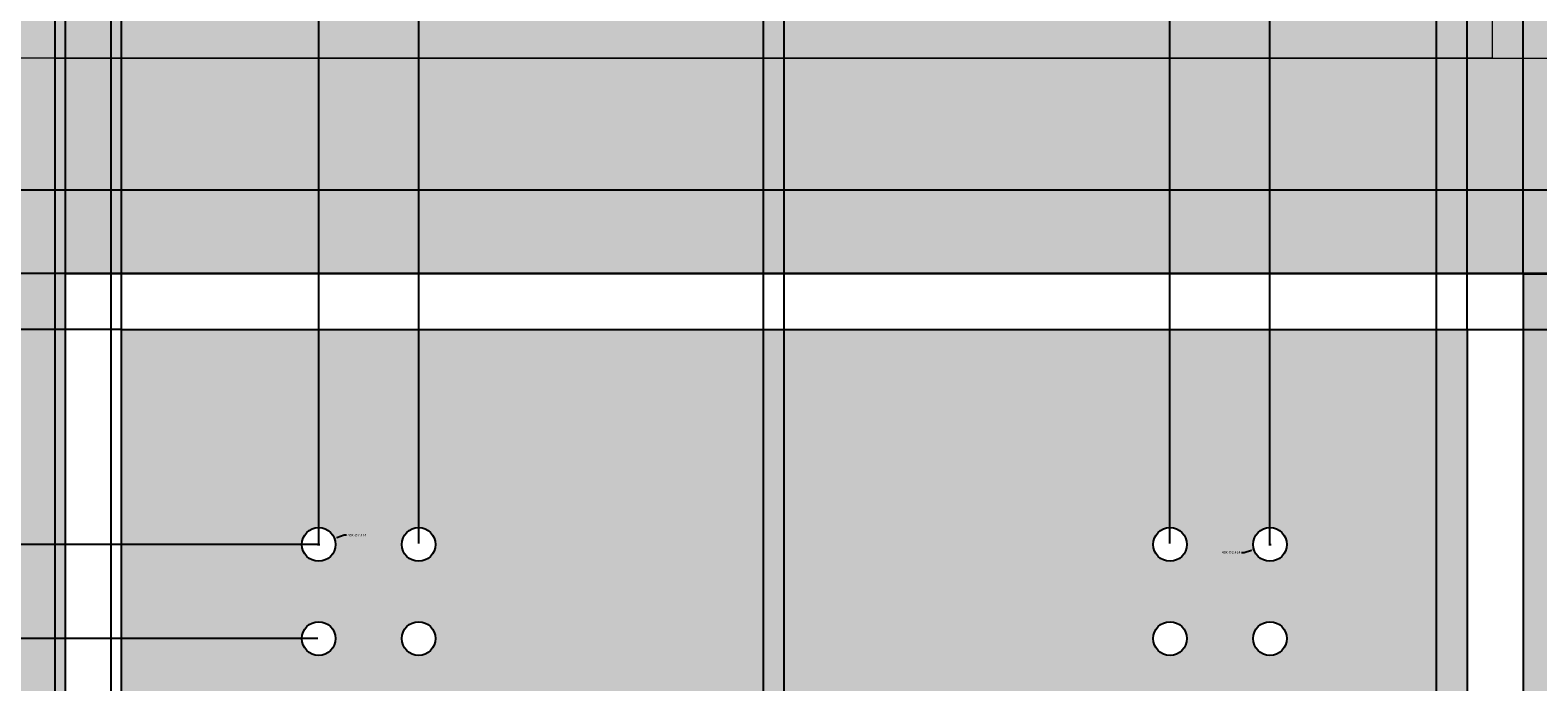
# Model space of a CAD drawing. Units: inches. Extents: x 3024 to 4744, y 1110 to 2100.
# Tile 6 of 29: x 3168 to 3275, y 1246 to 1293. Entities that reach past the tile are written whole.
import ezdxf

# ---------------------------------------------------------------- set-up
doc = ezdxf.new("R2010")
doc.units = ezdxf.units.IN
for name, color, linetype, lineweight in [('A-ANNO-DIMS', 2, 'Continuous', 18), ('A-ELEV', 7, 'Continuous', 25), ('A-ELEV-PATT', 252, 'Continuous', 13), ('A-GLAZ', 4, 'Continuous', 18)]:
    doc.layers.add(name, color=color, linetype=linetype, lineweight=lineweight)
doc.styles.get("Standard").update_dxf_attribs({"font": 'arial.ttf'})
doc.dimstyles.get("Standard").update_dxf_attribs({"dimtxt": 0.18, "dimasz": 0.18, "dimexe": 0.18, "dimexo": 0.0625, "dimgap": 0.09, "dimtad": 0, "dimtih": 1, "dimtoh": 1, "dimdec": 1, "dimzin": 0, "dimdsep": 46, "dimlunit": 3, "dimtxsty": 'Standard', "dimcen": 0.09, "dimadec": 0, "dimazin": 0, "dimtfac": 1, "dimtdec": 1, "dimtofl": 0, "dimtmove": 0, "dimatfit": 3, "dimfxl": 1, "dimtolj": 1, "dimtzin": 0, "dimarcsym": 0})

# ---------------------------------------------------------------- blocks, each defined once
blk = doc.blocks.new('WIN-BALCONY-A')
for q in [(3148.97, 1795.04), (3148.97, 1795.04), (3292.61, 1795.04), (3292.61, 1795.04)]:
    blk.add_line((3169.4, 1795.04), q)
blk.add_lwpolyline([(3272.18, 1795.04), (3169.4, 1795.04), (3169.4, 1897.49), (3272.18, 1897.49)], close=True)
blk.add_lwpolyline([(3272.18, 1795.04), (3169.4, 1795.04), (3169.4, 1897.49), (3272.18, 1897.49)], close=True)
blk.add_lwpolyline([(3292.61, 1795.04), (3292.61, 1785.61), (3148.97, 1785.61), (3148.97, 1795.04)])
blk.add_lwpolyline([(3292.61, 1795.04), (3292.61, 1785.61), (3148.97, 1785.61), (3148.97, 1795.04)])
blk = doc.blocks.new('*D52')
at = {"layer": 'A-ANNO-DIMS', "color": 0, "lineweight": -2, "transparency": 16777216}
for p, q in [((3148.97, 1290.98), (3148.97, 1109.93)), ((3170.16, 1170.96), (3170.16, 1109.93)), ((3149.15, 1110.11), (3159.17, 1110.11)), ((3169.98, 1110.11), (3159.96, 1110.11))]:
    blk.add_line(p, q, dxfattribs=at)
at = {"layer": 'A-ANNO-DIMS', "color": 0, "transparency": 16777216}
for points in [[(3149.15, 1110.14), (3149.15, 1110.08), (3148.97, 1110.11)], [(3169.98, 1110.14), (3169.98, 1110.08), (3170.16, 1110.11)]]:
    blk.add_solid(points, dxfattribs=at)
at = {"layer": 'Defpoints', "color": 0, "transparency": 16777216}
for p in [(3148.97, 1291.04), (3170.16, 1171.02), (3170.16, 1110.11)]:
    blk.add_point(p, dxfattribs=at)
at = {"layer": 'A-ANNO-DIMS', "color": 0, "transparency": 16777216, "insert": (3159.57, 1110.11), "char_height": 0.18, "attachment_point": 5}
blk.add_mtext('\\A1;21.19', dxfattribs=at)
blk = doc.blocks.new('*D54')
at = {"layer": 'A-ANNO-DIMS', "color": 0, "lineweight": -2, "transparency": 16777216}
for p, q in [((3292.61, 1290.98), (3292.61, 1109.93)), ((3274.39, 1170.96), (3274.39, 1109.93)), ((3274.57, 1110.11), (3283.04, 1110.11)), ((3292.43, 1110.11), (3283.95, 1110.11))]:
    blk.add_line(p, q, dxfattribs=at)
at = {"layer": 'A-ANNO-DIMS', "color": 0, "transparency": 16777216}
for points in [[(3274.57, 1110.14), (3274.57, 1110.08), (3274.39, 1110.11)], [(3292.43, 1110.14), (3292.43, 1110.08), (3292.61, 1110.11)]]:
    blk.add_solid(points, dxfattribs=at)
at = {"layer": 'Defpoints', "color": 0, "transparency": 16777216}
for p in [(3292.61, 1291.04), (3274.39, 1171.02), (3292.61, 1110.11)]:
    blk.add_point(p, dxfattribs=at)
at = {"layer": 'A-ANNO-DIMS', "color": 0, "transparency": 16777216, "insert": (3283.5, 1110.11), "char_height": 0.18, "attachment_point": 5}
blk.add_mtext('\\A1;18.217', dxfattribs=at)
blk = doc.blocks.new('*D64')
at = {"layer": 'A-ANNO-DIMS', "color": 0, "lineweight": -2, "transparency": 16777216}
for p, q in [((3069.79, 1241.5), (3069.79, 2100.44)), ((3741.15, 1241.5), (3741.15, 2100.44)), ((3069.97, 2100.26), (3405.08, 2100.26)), ((3740.97, 2100.26), (3405.87, 2100.26))]:
    blk.add_line(p, q, dxfattribs=at)
at = {"layer": 'A-ANNO-DIMS', "color": 0, "transparency": 16777216}
for points in [[(3069.97, 2100.29), (3069.97, 2100.23), (3069.79, 2100.26)], [(3740.97, 2100.29), (3740.97, 2100.23), (3741.15, 2100.26)]]:
    blk.add_solid(points, dxfattribs=at)
at = {"layer": 'Defpoints', "color": 0, "transparency": 16777216}
for p in [(3741.15, 2100.26), (3069.79, 1241.43), (3741.15, 1241.43)]:
    blk.add_point(p, dxfattribs=at)
at = {"layer": 'A-ANNO-DIMS', "color": 0, "transparency": 16777216, "insert": (3405.47, 2100.26), "char_height": 0.18, "attachment_point": 5}
blk.add_mtext('\\A1;671.4', dxfattribs=at)
blk = doc.blocks.new('*D77')
at = {"layer": 'A-ANNO-DIMS', "color": 0, "lineweight": -2, "transparency": 16777216}
for p, q in [((3188.17, 1256.23), (3188.35, 1256.23)), ((3188.26, 1256.14), (3188.26, 1256.32)), ((3190.07, 1256.89), (3189.56, 1256.71)), ((3190.25, 1256.89), (3190.07, 1256.89))]:
    blk.add_line(p, q, dxfattribs=at)
at = {"layer": 'A-ANNO-DIMS', "color": 0, "transparency": 16777216}
blk.add_solid([(3189.55, 1256.73), (3189.57, 1256.68), (3189.39, 1256.64)], dxfattribs=at)
at = {"layer": 'Defpoints', "color": 0, "transparency": 16777216}
for p in [(3189.39, 1256.64), (3187.13, 1255.81)]:
    blk.add_point(p, dxfattribs=at)
at = {"layer": 'A-ANNO-DIMS', "color": 0, "transparency": 16777216, "insert": (3191, 1256.89), "char_height": 0.18, "attachment_point": 5}
blk.add_mtext('\\A1;40X ∅2.414', dxfattribs=at)
blk = doc.blocks.new('*D90')
at = {"layer": 'A-ANNO-DIMS', "color": 0, "lineweight": -2, "transparency": 16777216}
for p, q in [((3173.4, 1798.98), (3173.4, 1109.93)), ((3169.4, 1794.98), (3169.4, 1109.93)), ((3169.58, 1110.11), (3171.07, 1110.11)), ((3173.22, 1110.11), (3171.72, 1110.11))]:
    blk.add_line(p, q, dxfattribs=at)
at = {"layer": 'A-ANNO-DIMS', "color": 0, "transparency": 16777216}
for points in [[(3169.58, 1110.14), (3169.58, 1110.08), (3169.4, 1110.11)], [(3173.22, 1110.14), (3173.22, 1110.08), (3173.4, 1110.11)]]:
    blk.add_solid(points, dxfattribs=at)
at = {"layer": 'Defpoints', "color": 0, "transparency": 16777216}
for p in [(3173.4, 1799.04), (3169.4, 1795.04), (3173.4, 1110.11)]:
    blk.add_point(p, dxfattribs=at)
at = {"layer": 'A-ANNO-DIMS', "color": 0, "transparency": 16777216, "insert": (3171.4, 1110.11), "char_height": 0.18, "attachment_point": 5}
blk.add_mtext('\\A1;4.00', dxfattribs=at)
blk = doc.blocks.new('*D91')
at = {"layer": 'A-ANNO-DIMS', "color": 0, "lineweight": -2, "transparency": 16777216}
for p, q in [((3173.4, 1798.98), (3173.4, 1109.93)), ((3220.05, 1798.98), (3220.05, 1109.93)), ((3173.58, 1110.11), (3196.33, 1110.11)), ((3219.87, 1110.11), (3197.12, 1110.11))]:
    blk.add_line(p, q, dxfattribs=at)
at = {"layer": 'A-ANNO-DIMS', "color": 0, "transparency": 16777216}
for points in [[(3173.58, 1110.14), (3173.58, 1110.08), (3173.4, 1110.11)], [(3219.87, 1110.14), (3219.87, 1110.08), (3220.05, 1110.11)]]:
    blk.add_solid(points, dxfattribs=at)
at = {"layer": 'Defpoints', "color": 0, "transparency": 16777216}
for p in [(3173.4, 1799.04), (3220.05, 1799.04), (3220.05, 1110.11)]:
    blk.add_point(p, dxfattribs=at)
at = {"layer": 'A-ANNO-DIMS', "color": 0, "transparency": 16777216, "insert": (3196.72, 1110.11), "char_height": 0.18, "attachment_point": 5}
blk.add_mtext('\\A1;46.65', dxfattribs=at)
blk = doc.blocks.new('*D92')
at = {"layer": 'A-ANNO-DIMS', "color": 0, "lineweight": -2, "transparency": 16777216}
for p, q in [((3220.05, 1798.98), (3220.05, 1109.93)), ((3221.52, 1798.98), (3221.52, 1109.93)), ((3220.23, 1110.11), (3220.47, 1110.11)), ((3221.34, 1110.11), (3221.1, 1110.11))]:
    blk.add_line(p, q, dxfattribs=at)
at = {"layer": 'A-ANNO-DIMS', "color": 0, "transparency": 16777216}
for points in [[(3220.23, 1110.14), (3220.23, 1110.08), (3220.05, 1110.11)], [(3221.34, 1110.14), (3221.34, 1110.08), (3221.52, 1110.11)]]:
    blk.add_solid(points, dxfattribs=at)
at = {"layer": 'Defpoints', "color": 0, "transparency": 16777216}
for p in [(3220.05, 1799.04), (3221.52, 1799.04), (3221.52, 1110.11)]:
    blk.add_point(p, dxfattribs=at)
at = {"layer": 'A-ANNO-DIMS', "color": 0, "transparency": 16777216, "insert": (3220.79, 1110.11), "char_height": 0.18, "attachment_point": 5}
blk.add_mtext('\\A1;1.47', dxfattribs=at)
blk = doc.blocks.new('*D93')
at = {"layer": 'A-ANNO-DIMS', "color": 0, "lineweight": -2, "transparency": 16777216}
for p, q in [((3221.52, 1798.98), (3221.52, 1109.93)), ((3268.18, 1798.98), (3268.18, 1109.93)), ((3221.7, 1110.11), (3244.45, 1110.11)), ((3268, 1110.11), (3245.25, 1110.11))]:
    blk.add_line(p, q, dxfattribs=at)
at = {"layer": 'A-ANNO-DIMS', "color": 0, "transparency": 16777216}
for points in [[(3221.7, 1110.14), (3221.7, 1110.08), (3221.52, 1110.11)], [(3268, 1110.14), (3268, 1110.08), (3268.18, 1110.11)]]:
    blk.add_solid(points, dxfattribs=at)
at = {"layer": 'Defpoints', "color": 0, "transparency": 16777216}
for p in [(3221.52, 1799.04), (3268.18, 1799.04), (3268.18, 1110.11)]:
    blk.add_point(p, dxfattribs=at)
at = {"layer": 'A-ANNO-DIMS', "color": 0, "transparency": 16777216, "insert": (3244.85, 1110.11), "char_height": 0.18, "attachment_point": 5}
blk.add_mtext('\\A1;46.65', dxfattribs=at)
blk = doc.blocks.new('*D106')
at = {"layer": 'A-ANNO-DIMS', "color": 0, "lineweight": -2, "transparency": 16777216}
for p, q in [((3170.16, 1275.67), (3170.16, 2100.44)), ((3174.16, 1271.67), (3174.16, 2100.44)), ((3170.34, 2100.26), (3171.83, 2100.26)), ((3173.98, 2100.26), (3172.49, 2100.26))]:
    blk.add_line(p, q, dxfattribs=at)
at = {"layer": 'A-ANNO-DIMS', "color": 0, "transparency": 16777216}
for points in [[(3170.34, 2100.29), (3170.34, 2100.23), (3170.16, 2100.26)], [(3173.98, 2100.29), (3173.98, 2100.23), (3174.16, 2100.26)]]:
    blk.add_solid(points, dxfattribs=at)
at = {"layer": 'Defpoints', "color": 0, "transparency": 16777216}
for p in [(3174.16, 2100.26), (3170.16, 1275.61), (3174.16, 1271.61)]:
    blk.add_point(p, dxfattribs=at)
at = {"layer": 'A-ANNO-DIMS', "color": 0, "transparency": 16777216, "insert": (3172.16, 2100.26), "char_height": 0.18, "attachment_point": 5}
blk.add_mtext('\\A1;4.00', dxfattribs=at)
blk = doc.blocks.new('*D107')
at = {"layer": 'A-ANNO-DIMS', "color": 0, "lineweight": -2, "transparency": 16777216}
for p, q in [((3174.16, 1271.67), (3174.16, 2100.44)), ((3270.39, 1271.67), (3270.39, 2100.44)), ((3174.34, 2100.26), (3221.88, 2100.26)), ((3270.21, 2100.26), (3222.67, 2100.26))]:
    blk.add_line(p, q, dxfattribs=at)
at = {"layer": 'A-ANNO-DIMS', "color": 0, "transparency": 16777216}
for points in [[(3174.34, 2100.29), (3174.34, 2100.23), (3174.16, 2100.26)], [(3270.21, 2100.29), (3270.21, 2100.23), (3270.39, 2100.26)]]:
    blk.add_solid(points, dxfattribs=at)
at = {"layer": 'Defpoints', "color": 0, "transparency": 16777216}
for p in [(3270.39, 2100.26), (3174.16, 1271.61), (3270.39, 1271.61)]:
    blk.add_point(p, dxfattribs=at)
at = {"layer": 'A-ANNO-DIMS', "color": 0, "transparency": 16777216, "insert": (3222.27, 2100.26), "char_height": 0.18, "attachment_point": 5}
blk.add_mtext('\\A1;96.23', dxfattribs=at)
blk = doc.blocks.new('*D108')
at = {"layer": 'A-ANNO-DIMS', "color": 0, "lineweight": -2, "transparency": 16777216}
for p, q in [((3270.39, 1271.67), (3270.39, 2100.44)), ((3274.39, 1275.67), (3274.39, 2100.44)), ((3270.57, 2100.26), (3272.06, 2100.26)), ((3274.21, 2100.26), (3272.71, 2100.26))]:
    blk.add_line(p, q, dxfattribs=at)
at = {"layer": 'A-ANNO-DIMS', "color": 0, "transparency": 16777216}
for points in [[(3270.57, 2100.29), (3270.57, 2100.23), (3270.39, 2100.26)], [(3274.21, 2100.29), (3274.21, 2100.23), (3274.39, 2100.26)]]:
    blk.add_solid(points, dxfattribs=at)
at = {"layer": 'Defpoints', "color": 0, "transparency": 16777216}
for p in [(3274.39, 2100.26), (3274.39, 1275.61), (3270.39, 1271.61)]:
    blk.add_point(p, dxfattribs=at)
at = {"layer": 'A-ANNO-DIMS', "color": 0, "transparency": 16777216, "insert": (3272.39, 2100.26), "char_height": 0.18, "attachment_point": 5}
blk.add_mtext('\\A1;4.00', dxfattribs=at)
blk = doc.blocks.new('*D120')
at = {"layer": 'A-ANNO-DIMS', "color": 0, "lineweight": -2, "transparency": 16777216}
for p, q in [((3270.45, 1271.61), (3786.83, 1271.61)), ((3786.65, 1271.43), (3786.65, 1221.5)), ((3786.65, 1171.2), (3786.65, 1221.14)), ((3274.45, 1171.02), (3786.83, 1171.02))]:
    blk.add_line(p, q, dxfattribs=at)
at = {"layer": 'A-ANNO-DIMS', "color": 0, "transparency": 16777216}
for points in [[(3786.62, 1271.43), (3786.68, 1271.43), (3786.65, 1271.61)], [(3786.62, 1171.2), (3786.68, 1171.2), (3786.65, 1171.02)]]:
    blk.add_solid(points, dxfattribs=at)
at = {"layer": 'Defpoints', "color": 0, "transparency": 16777216}
for p in [(3270.39, 1271.61), (3786.65, 1271.61), (3274.39, 1171.02)]:
    blk.add_point(p, dxfattribs=at)
at = {"layer": 'A-ANNO-DIMS', "color": 0, "transparency": 16777216, "insert": (3786.65, 1221.32), "char_height": 0.18, "attachment_point": 5}
blk.add_mtext('\\A1;100.59', dxfattribs=at)
blk = doc.blocks.new('*D121')
at = {"layer": 'A-ANNO-DIMS', "color": 0, "lineweight": -2, "transparency": 16777216}
for p, q in [((3274.45, 1275.61), (3786.83, 1275.61)), ((3786.65, 1275.43), (3786.65, 1273.79)), ((3786.65, 1271.79), (3786.65, 1273.43)), ((3270.45, 1271.61), (3786.83, 1271.61))]:
    blk.add_line(p, q, dxfattribs=at)
at = {"layer": 'A-ANNO-DIMS', "color": 0, "transparency": 16777216}
for points in [[(3786.62, 1275.43), (3786.68, 1275.43), (3786.65, 1275.61)], [(3786.62, 1271.79), (3786.68, 1271.79), (3786.65, 1271.61)]]:
    blk.add_solid(points, dxfattribs=at)
at = {"layer": 'Defpoints', "color": 0, "transparency": 16777216}
for p in [(3274.39, 1275.61), (3786.65, 1275.61), (3270.39, 1271.61)]:
    blk.add_point(p, dxfattribs=at)
at = {"layer": 'A-ANNO-DIMS', "color": 0, "transparency": 16777216, "insert": (3786.65, 1273.61), "char_height": 0.18, "attachment_point": 5}
blk.add_mtext('\\A1;4.00', dxfattribs=at)
blk = doc.blocks.new('*D124')
at = {"layer": 'A-ANNO-DIMS', "color": 0, "lineweight": -2, "transparency": 16777216}
for p, q in [((3174.16, 1271.67), (3174.16, 2100.44)), ((3188.26, 1256.29), (3188.26, 2100.44)), ((3174.34, 2100.26), (3180.75, 2100.26)), ((3188.08, 2100.26), (3181.67, 2100.26))]:
    blk.add_line(p, q, dxfattribs=at)
at = {"layer": 'A-ANNO-DIMS', "color": 0, "transparency": 16777216}
for points in [[(3174.34, 2100.29), (3174.34, 2100.23), (3174.16, 2100.26)], [(3188.08, 2100.29), (3188.08, 2100.23), (3188.26, 2100.26)]]:
    blk.add_solid(points, dxfattribs=at)
at = {"layer": 'Defpoints', "color": 0, "transparency": 16777216}
for p in [(3188.26, 2100.26), (3174.16, 1271.61), (3188.26, 1256.23)]:
    blk.add_point(p, dxfattribs=at)
at = {"layer": 'A-ANNO-DIMS', "color": 0, "transparency": 16777216, "insert": (3181.21, 2100.26), "char_height": 0.18, "attachment_point": 5}
blk.add_mtext('\\A1;14.098', dxfattribs=at)
blk = doc.blocks.new('*D125')
at = {"layer": 'A-ANNO-DIMS', "color": 0, "lineweight": -2, "transparency": 16777216}
for p, q in [((3188.26, 1256.29), (3188.26, 2100.44)), ((3195.41, 1256.29), (3195.41, 2100.44)), ((3188.44, 2100.26), (3191.44, 2100.26)), ((3195.23, 2100.26), (3192.22, 2100.26))]:
    blk.add_line(p, q, dxfattribs=at)
at = {"layer": 'A-ANNO-DIMS', "color": 0, "transparency": 16777216}
for points in [[(3188.44, 2100.29), (3188.44, 2100.23), (3188.26, 2100.26)], [(3195.23, 2100.29), (3195.23, 2100.23), (3195.41, 2100.26)]]:
    blk.add_solid(points, dxfattribs=at)
at = {"layer": 'Defpoints', "color": 0, "transparency": 16777216}
for p in [(3195.41, 2100.26), (3188.26, 1256.23), (3195.41, 1256.23)]:
    blk.add_point(p, dxfattribs=at)
at = {"layer": 'A-ANNO-DIMS', "color": 0, "transparency": 16777216, "insert": (3191.83, 2100.26), "char_height": 0.18, "attachment_point": 5}
blk.add_mtext('\\A1;7.147', dxfattribs=at)
blk = doc.blocks.new('*D126')
at = {"layer": 'A-ANNO-DIMS', "color": 0, "lineweight": -2, "transparency": 16777216}
for p, q in [((3249.14, 1256.29), (3249.14, 2100.44)), ((3256.29, 1256.29), (3256.29, 2100.44)), ((3249.32, 2100.26), (3252.32, 2100.26)), ((3256.11, 2100.26), (3253.11, 2100.26))]:
    blk.add_line(p, q, dxfattribs=at)
at = {"layer": 'A-ANNO-DIMS', "color": 0, "transparency": 16777216}
for points in [[(3249.32, 2100.29), (3249.32, 2100.23), (3249.14, 2100.26)], [(3256.11, 2100.29), (3256.11, 2100.23), (3256.29, 2100.26)]]:
    blk.add_solid(points, dxfattribs=at)
at = {"layer": 'Defpoints', "color": 0, "transparency": 16777216}
for p in [(3256.29, 2100.26), (3249.14, 1256.23), (3256.29, 1256.23)]:
    blk.add_point(p, dxfattribs=at)
at = {"layer": 'A-ANNO-DIMS', "color": 0, "transparency": 16777216, "insert": (3252.72, 2100.26), "char_height": 0.18, "attachment_point": 5}
blk.add_mtext('\\A1;7.147', dxfattribs=at)
blk = doc.blocks.new('*D127')
at = {"layer": 'A-ANNO-DIMS', "color": 0, "lineweight": -2, "transparency": 16777216}
for p, q in [((3174.1, 1271.61), (3024.11, 1271.61)), ((3024.29, 1271.43), (3024.29, 1264.1)), ((3024.29, 1256.41), (3024.29, 1263.74)), ((3188.2, 1256.23), (3024.11, 1256.23))]:
    blk.add_line(p, q, dxfattribs=at)
at = {"layer": 'A-ANNO-DIMS', "color": 0, "transparency": 16777216}
for points in [[(3024.26, 1271.43), (3024.32, 1271.43), (3024.29, 1271.61)], [(3024.26, 1256.41), (3024.32, 1256.41), (3024.29, 1256.23)]]:
    blk.add_solid(points, dxfattribs=at)
at = {"layer": 'Defpoints', "color": 0, "transparency": 16777216}
for p in [(3174.16, 1271.61), (3024.29, 1256.23), (3188.26, 1256.23)]:
    blk.add_point(p, dxfattribs=at)
at = {"layer": 'A-ANNO-DIMS', "color": 0, "transparency": 16777216, "insert": (3024.29, 1263.92), "char_height": 0.18, "attachment_point": 5}
blk.add_mtext('\\A1;15.384', dxfattribs=at)
blk = doc.blocks.new('*D128')
at = {"layer": 'A-ANNO-DIMS', "color": 0, "lineweight": -2, "transparency": 16777216}
for p, q in [((3188.2, 1256.23), (3024.11, 1256.23)), ((3024.29, 1256.05), (3024.29, 1253.04)), ((3024.29, 1249.67), (3024.29, 1252.68)), ((3188.2, 1249.49), (3024.11, 1249.49))]:
    blk.add_line(p, q, dxfattribs=at)
at = {"layer": 'A-ANNO-DIMS', "color": 0, "transparency": 16777216}
for points in [[(3024.26, 1256.05), (3024.32, 1256.05), (3024.29, 1256.23)], [(3024.26, 1249.67), (3024.32, 1249.67), (3024.29, 1249.49)]]:
    blk.add_solid(points, dxfattribs=at)
at = {"layer": 'Defpoints', "color": 0, "transparency": 16777216}
for p in [(3188.26, 1256.23), (3024.29, 1249.49), (3188.26, 1249.49)]:
    blk.add_point(p, dxfattribs=at)
at = {"layer": 'A-ANNO-DIMS', "color": 0, "transparency": 16777216, "insert": (3024.29, 1252.86), "char_height": 0.18, "attachment_point": 5}
blk.add_mtext('\\A1;6.738', dxfattribs=at)
blk = doc.blocks.new('*D129')
at = {"layer": 'A-ANNO-DIMS', "color": 0, "lineweight": -2, "transparency": 16777216}
for p, q in [((3188.2, 1249.49), (3024.11, 1249.49)), ((3024.29, 1249.31), (3024.29, 1243.37)), ((3024.29, 1237.07), (3024.29, 1243.01)), ((3188.2, 1236.89), (3024.11, 1236.89))]:
    blk.add_line(p, q, dxfattribs=at)
at = {"layer": 'A-ANNO-DIMS', "color": 0, "transparency": 16777216}
for points in [[(3024.26, 1249.31), (3024.32, 1249.31), (3024.29, 1249.49)], [(3024.26, 1237.07), (3024.32, 1237.07), (3024.29, 1236.89)]]:
    blk.add_solid(points, dxfattribs=at)
at = {"layer": 'Defpoints', "color": 0, "transparency": 16777216}
for p in [(3188.26, 1249.49), (3024.29, 1236.89), (3188.26, 1236.89)]:
    blk.add_point(p, dxfattribs=at)
at = {"layer": 'A-ANNO-DIMS', "color": 0, "transparency": 16777216, "insert": (3024.29, 1243.19), "char_height": 0.18, "attachment_point": 5}
blk.add_mtext('\\A1;12.603', dxfattribs=at)
blk = doc.blocks.new('*D131')
at = {"layer": 'A-ANNO-DIMS', "color": 0, "lineweight": -2, "transparency": 16777216}
for p, q in [((3256.2, 1256.23), (3256.38, 1256.23)), ((3256.29, 1256.14), (3256.29, 1256.32)), ((3254.26, 1255.66), (3254.44, 1255.66)), ((3254.44, 1255.66), (3254.96, 1255.82))]:
    blk.add_line(p, q, dxfattribs=at)
at = {"layer": 'A-ANNO-DIMS', "color": 0, "transparency": 16777216}
blk.add_solid([(3254.95, 1255.85), (3254.97, 1255.79), (3255.14, 1255.87)], dxfattribs=at)
at = {"layer": 'Defpoints', "color": 0, "transparency": 16777216}
for p in [(3257.44, 1256.58), (3255.14, 1255.87)]:
    blk.add_point(p, dxfattribs=at)
at = {"layer": 'A-ANNO-DIMS', "color": 0, "transparency": 16777216, "insert": (3253.51, 1255.66), "char_height": 0.18, "attachment_point": 5}
blk.add_mtext('\\A1;40X ∅2.414', dxfattribs=at)

msp = doc.modelspace()

# ---------------------------------------------------------------- hatches: boundary and pattern name
at = {"layer": 'A-ELEV-PATT'}
h = msp.add_hatch(color=256, dxfattribs=at)
h.dxf.hatch_style = 1
h.paths.add_polyline_path([(3491.8271, 2054.7584), (3320.5658, 2054.7584), (3320.5658, 2043.5286), (3491.8271, 2043.5286)])
h.paths.add_polyline_path([(3292.6051, 1905.6112), (3148.9694, 1905.6112), (3148.9694, 1897.4879), (3169.3964, 1897.4879), (3292.6051, 1897.4879)])
h.paths.add_polyline_path([(3292.6051, 1795.0431), (3169.3964, 1795.0431), (3148.9694, 1795.0431), (3148.9694, 1785.6112), (3292.6051, 1785.6112)])
h.paths.add_polyline_path([(3292.6051, 1779.6112), (3148.9694, 1779.6112), (3148.9694, 1771.4879), (3169.3964, 1771.4879), (3292.6051, 1771.4879)])
h.paths.add_polyline_path([(3292.6051, 1669.0431), (3169.3964, 1669.0431), (3148.9694, 1669.0431), (3148.9694, 1659.6112), (3292.6051, 1659.6112)])
h.paths.add_polyline_path([(3292.6051, 1653.6112), (3148.9694, 1653.6112), (3148.9694, 1645.4879), (3169.3964, 1645.4879), (3292.6051, 1645.4879)])
h.paths.add_polyline_path([(3292.6051, 1543.0431), (3169.3964, 1543.0431), (3148.9694, 1543.0431), (3148.9694, 1533.6112), (3292.6051, 1533.6112)])
h.paths.add_polyline_path([(3292.6051, 1527.6112), (3148.9694, 1527.6112), (3148.9694, 1519.4879), (3169.3964, 1519.4879), (3292.6051, 1519.4879)])
h.paths.add_polyline_path([(3292.6051, 1401.6112), (3148.9694, 1401.6112), (3148.9694, 1393.4879), (3169.3964, 1393.4879), (3292.6051, 1393.4879)])
h.paths.add_polyline_path([(3292.6051, 1417.0431), (3169.3964, 1417.0431), (3148.9694, 1417.0431), (3148.9694, 1407.6112), (3292.6051, 1407.6112)])
h.paths.add_polyline_path([(3292.6051, 1291.0431), (3169.3964, 1291.0431), (3148.9694, 1291.0431), (3148.9694, 1281.6112), (3292.6051, 1281.6112)])
h.paths.add_polyline_path([(3654.037, 1165.0431), (3530.8283, 1165.0431), (3510.4013, 1165.0431), (3510.4013, 1155.6112), (3654.037, 1155.6112)])
h.paths.add_polyline_path([(3654.037, 1275.6112), (3510.4013, 1275.6112), (3510.4013, 1267.4879), (3530.8283, 1267.4879), (3654.037, 1267.4879)])
h.paths.add_polyline_path([(3654.037, 1291.0431), (3530.8283, 1291.0431), (3510.4013, 1291.0431), (3510.4013, 1281.6112), (3654.037, 1281.6112)])
h.paths.add_polyline_path([(3654.037, 1417.0431), (3530.8283, 1417.0431), (3510.4013, 1417.0431), (3510.4013, 1407.6112), (3654.037, 1407.6112)])
h.paths.add_polyline_path([(3654.037, 1401.6112), (3510.4013, 1401.6112), (3510.4013, 1393.4879), (3530.8283, 1393.4879), (3654.037, 1393.4879)])
h.paths.add_polyline_path([(3654.037, 1543.0431), (3530.8283, 1543.0431), (3510.4013, 1543.0431), (3510.4013, 1533.6112), (3654.037, 1533.6112)])
h.paths.add_polyline_path([(3654.037, 1527.6112), (3510.4013, 1527.6112), (3510.4013, 1519.4879), (3530.8283, 1519.4879), (3654.037, 1519.4879)])
h.paths.add_polyline_path([(3654.037, 1653.6112), (3510.4013, 1653.6112), (3510.4013, 1645.4879), (3530.8283, 1645.4879), (3654.037, 1645.4879)])
h.paths.add_polyline_path([(3654.037, 1669.0431), (3530.8283, 1669.0431), (3510.4013, 1669.0431), (3510.4013, 1659.6112), (3654.037, 1659.6112)])
h.paths.add_polyline_path([(3654.037, 1779.6112), (3510.4013, 1779.6112), (3510.4013, 1771.4879), (3530.8283, 1771.4879), (3654.037, 1771.4879)])
h.paths.add_polyline_path([(3654.037, 1795.0431), (3530.8283, 1795.0431), (3510.4013, 1795.0431), (3510.4013, 1785.6112), (3654.037, 1785.6112)])
h.paths.add_polyline_path([(3654.037, 1905.6112), (3510.4013, 1905.6112), (3510.4013, 1897.4879), (3530.8283, 1897.4879), (3654.037, 1897.4879)])
h = msp.add_hatch(color=256, dxfattribs=at)
h.dxf.hatch_style = 1
h.paths.add_polyline_path([(3329.7033, 1407.6112), (3105.4722, 1407.6112), (3105.4722, 1401.6112), (3329.7033, 1401.6112)])
h.paths.add_polyline_path([(3329.7033, 1281.6112), (3105.4722, 1281.6112), (3105.4722, 1275.6112), (3112.3838, 1275.6112), (3329.7033, 1275.6112)])
h.paths.add_polyline_path([(3329.7033, 1533.6112), (3105.4722, 1533.6112), (3105.4722, 1527.6112), (3329.7033, 1527.6112)])
h.paths.add_polyline_path([(3329.7033, 1659.6112), (3105.4722, 1659.6112), (3105.4722, 1653.6112), (3329.7033, 1653.6112)])
h.paths.add_polyline_path([(3329.7033, 1785.6112), (3105.4722, 1785.6112), (3105.4722, 1779.6112), (3329.7033, 1779.6112)])
h.paths.add_polyline_path([(3329.7033, 1911.6112), (3105.4722, 1911.6112), (3095.7158, 1911.6112), (3095.7158, 1905.6112), (3329.7033, 1905.6112)])
h.paths.add_polyline_path([(3715.2286, 1911.6112), (3705.4722, 1911.6112), (3705.4722, 1905.6112), (3715.2286, 1905.6112)])
h.paths.add_polyline_path([(3688.5588, 1911.6112), (3481.2411, 1911.6112), (3481.2411, 1905.6112), (3688.5588, 1905.6112)])
h = msp.add_hatch(color=256, dxfattribs=at)
h.dxf.hatch_style = 1
h.paths.add_polyline_path([(3169.3964, 1897.4879), (3160.8586, 1897.4879), (3160.8586, 1806.8674), (3163.5269, 1806.8674), (3163.5269, 1795.0431), (3169.3964, 1795.0431)])
h.paths.add_polyline_path([(3280.716, 1897.4879), (3272.1781, 1897.4879), (3272.1781, 1795.0431), (3276.5094, 1795.0431), (3276.5094, 1806.8674), (3280.716, 1806.8674)])
h.paths.add_polyline_path([(3280.716, 1771.4879), (3272.1781, 1771.4879), (3272.1781, 1669.0431), (3276.5094, 1669.0431), (3276.5094, 1680.8674), (3280.716, 1680.8674)])
h.paths.add_polyline_path([(3169.3964, 1771.4879), (3160.8586, 1771.4879), (3160.8586, 1680.8674), (3163.5269, 1680.8674), (3163.5269, 1669.0431), (3169.3964, 1669.0431)])
h.paths.add_polyline_path([(3169.3964, 1645.4879), (3160.8586, 1645.4879), (3160.8586, 1554.8674), (3163.5269, 1554.8674), (3163.5269, 1543.0431), (3169.3964, 1543.0431)])
h.paths.add_polyline_path([(3280.716, 1645.4879), (3272.1781, 1645.4879), (3272.1781, 1543.0431), (3276.5094, 1543.0431), (3276.5094, 1554.8674), (3280.716, 1554.8674)])
h.paths.add_polyline_path([(3169.3964, 1519.4879), (3160.8586, 1519.4879), (3160.8586, 1428.8674), (3163.5269, 1428.8674), (3163.5269, 1417.0431), (3169.3964, 1417.0431)])
h.paths.add_polyline_path([(3280.716, 1519.4879), (3272.1781, 1519.4879), (3272.1781, 1417.0431), (3276.5094, 1417.0431), (3276.5094, 1428.8674), (3280.716, 1428.8674)])
h.paths.add_polyline_path([(3169.3964, 1393.4879), (3160.8586, 1393.4879), (3160.8586, 1302.8674), (3163.5269, 1302.8674), (3163.5269, 1291.0431), (3169.3964, 1291.0431)])
h.paths.add_polyline_path([(3280.716, 1393.4879), (3272.1781, 1393.4879), (3272.1781, 1291.0431), (3276.5094, 1291.0431), (3276.5094, 1302.8674), (3280.716, 1302.8674)])
h.paths.add_polyline_path([(3642.1479, 1267.4879), (3633.61, 1267.4879), (3633.61, 1165.0431), (3637.9413, 1165.0431), (3637.9413, 1176.8674), (3642.1479, 1176.8674)])
h.paths.add_polyline_path([(3530.8283, 1267.4879), (3522.2905, 1267.4879), (3522.2905, 1176.8674), (3524.9588, 1176.8674), (3524.9588, 1165.0431), (3530.8283, 1165.0431)])
h.paths.add_polyline_path([(3642.1479, 1393.4879), (3633.61, 1393.4879), (3633.61, 1291.0431), (3637.9413, 1291.0431), (3637.9413, 1302.8674), (3642.1479, 1302.8674)])
h.paths.add_polyline_path([(3530.8283, 1393.4879), (3522.2905, 1393.4879), (3522.2905, 1302.8674), (3524.9588, 1302.8674), (3524.9588, 1291.0431), (3530.8283, 1291.0431)])
h.paths.add_polyline_path([(3530.8283, 1519.4879), (3522.2905, 1519.4879), (3522.2905, 1428.8674), (3524.9588, 1428.8674), (3524.9588, 1417.0431), (3530.8283, 1417.0431)])
h.paths.add_polyline_path([(3642.1479, 1519.4879), (3633.61, 1519.4879), (3633.61, 1417.0431), (3637.9413, 1417.0431), (3637.9413, 1428.8674), (3642.1479, 1428.8674)])
h.paths.add_polyline_path([(3530.8283, 1645.4879), (3522.2905, 1645.4879), (3522.2905, 1554.8674), (3524.9588, 1554.8674), (3524.9588, 1543.0431), (3530.8283, 1543.0431)])
h.paths.add_polyline_path([(3642.1479, 1645.4879), (3633.61, 1645.4879), (3633.61, 1543.0431), (3637.9413, 1543.0431), (3637.9413, 1554.8674), (3642.1479, 1554.8674)])
h.paths.add_polyline_path([(3642.1479, 1771.4879), (3633.61, 1771.4879), (3633.61, 1669.0431), (3637.9413, 1669.0431), (3637.9413, 1680.8674), (3642.1479, 1680.8674)])
h.paths.add_polyline_path([(3530.8283, 1771.4879), (3522.2905, 1771.4879), (3522.2905, 1680.8674), (3524.9588, 1680.8674), (3524.9588, 1669.0431), (3530.8283, 1669.0431)])
h.paths.add_polyline_path([(3530.8283, 1897.4879), (3522.2905, 1897.4879), (3522.2905, 1806.8674), (3524.9588, 1806.8674), (3524.9588, 1795.0431), (3530.8283, 1795.0431)])
h.paths.add_polyline_path([(3642.1479, 1897.4879), (3633.61, 1897.4879), (3633.61, 1795.0431), (3637.9413, 1795.0431), (3637.9413, 1806.8674), (3642.1479, 1806.8674)])
h = msp.add_hatch(color=256, dxfattribs=at)
h.dxf.hatch_style = 1
h.paths.add_polyline_path([(3221.5241, 1389.4879), (3220.0505, 1389.4879), (3220.0505, 1295.0431), (3221.5241, 1295.0431)], flags=0)
h.paths.add_polyline_path([(3272.1781, 1393.4879), (3169.3964, 1393.4879), (3169.3964, 1291.0431), (3272.1781, 1291.0431)])
h.paths.add_polyline_path([(3268.1781, 1389.4879), (3268.1781, 1295.0431), (3173.3964, 1295.0431), (3173.3964, 1389.4879)], flags=16)
h.paths.add_polyline_path([(3221.5241, 1389.4879), (3221.5241, 1295.0431), (3220.0505, 1295.0431), (3220.0505, 1389.4879)], flags=0)
h = msp.add_hatch(color=256, dxfattribs=at)
h.dxf.hatch_style = 1
h.paths.add_polyline_path([(3329.7033, 1275.6112), (3274.3877, 1275.6112), (3274.3877, 1171.0239), (3329.7033, 1171.0239)])
h.paths.add_polyline_path([(3323.3693, 1246.0161), (3279.3584, 1246.0161), (3279.3584, 1270.5642), (3323.3693, 1270.5642)], flags=16)
h.paths.add_polyline_path([(3323.3693, 1238.118), (3323.3693, 1213.5699), (3279.3584, 1213.5699), (3279.3584, 1238.118)], flags=16)
h.paths.add_polyline_path([(3323.3693, 1205.6718), (3323.3693, 1181.1236), (3279.3584, 1181.1236), (3279.3584, 1205.6718)], flags=16)
h.paths.add_polyline_path([(3170.1608, 1275.6112), (3112.3838, 1275.6112), (3112.3838, 1171.0239), (3118.1176, 1171.0239), (3170.1608, 1171.0239)])
h.paths.add_polyline_path([(3120.3696, 1246.0161), (3120.3696, 1270.5642), (3164.3806, 1270.5642), (3164.3806, 1246.0161)], flags=16)
h.paths.add_polyline_path([(3120.3696, 1238.118), (3164.3806, 1238.118), (3164.3806, 1213.5699), (3120.3696, 1213.5699)], flags=16)
h.paths.add_polyline_path([(3120.3696, 1205.6718), (3164.3806, 1205.6718), (3164.3806, 1181.1236), (3120.3696, 1181.1236)], flags=16)
h = msp.add_hatch(color=256, dxfattribs=at)
h.dxf.hatch_style = 1
h.paths.add_polyline_path([(3270.3877, 1271.6112), (3174.1608, 1271.6112), (3174.1608, 1171.0239), (3187.7692, 1171.0239, -0.29659686), (3187.0515, 1172.1274, -1), (3189.4658, 1172.1274, -0.29659686), (3188.7481, 1171.0239), (3194.9159, 1171.0239, -0.29659686), (3194.1982, 1172.1274, -1), (3196.6124, 1172.1274, -0.29659686), (3195.8947, 1171.0239), (3248.6539, 1171.0239, -0.29659686), (3247.9362, 1172.1274, -1), (3250.3504, 1172.1274, -0.29659686), (3249.6327, 1171.0239), (3255.8005, 1171.0239, -0.29659686), (3255.0828, 1172.1274, -1), (3257.4971, 1172.1274, -0.29659686), (3256.7794, 1171.0239), (3270.3877, 1171.0239)])
h.paths.add_polyline_path([(3196.6124, 1256.2276, -1), (3194.1982, 1256.2276, -1)], flags=16)
h.paths.add_polyline_path([(3196.6124, 1249.4899, -1), (3194.1982, 1249.4899, -1)], flags=16)
h.paths.add_polyline_path([(3216.163, 1245.2708), (3228.3856, 1245.2708), (3228.3856, 1185.9515), (3216.163, 1185.9515)], flags=16)
h.paths.add_polyline_path([(3187.0515, 1256.2276, -1), (3189.4658, 1256.2276, -1)], flags=16)
h.paths.add_polyline_path([(3189.4658, 1249.4899, -1), (3187.0515, 1249.4899, -1)], flags=16)
h.paths.add_polyline_path([(3196.6124, 1236.8869, -1), (3194.1982, 1236.8869, -1)], flags=16)
h.paths.add_polyline_path([(3189.4658, 1236.8869, -1), (3187.0515, 1236.8869, -1)], flags=16)
h.paths.add_polyline_path([(3196.6124, 1230.1493, -1), (3194.1982, 1230.1493, -1)], flags=16)
h.paths.add_polyline_path([(3189.4658, 1230.1493, -1), (3187.0515, 1230.1493, -1)], flags=16)
h.paths.add_polyline_path([(3250.3504, 1256.2276, -1), (3247.9362, 1256.2276, -1)], flags=16)
h.paths.add_polyline_path([(3250.3504, 1249.4899, -1), (3247.9362, 1249.4899, -1)], flags=16)
h.paths.add_polyline_path([(3196.6124, 1217.5463, -1), (3194.1982, 1217.5463, -1)], flags=16)
h.paths.add_polyline_path([(3250.3504, 1236.8869, -1), (3247.9362, 1236.8869, -1)], flags=16)
h.paths.add_polyline_path([(3189.4658, 1217.5463, -1), (3187.0515, 1217.5463, -1)], flags=16)
h.paths.add_polyline_path([(3257.4971, 1256.2276, -1), (3255.0828, 1256.2276, -1)], flags=16)
h.paths.add_polyline_path([(3257.4971, 1249.4899, -1), (3255.0828, 1249.4899, -1)], flags=16)
h.paths.add_polyline_path([(3250.3504, 1230.1493, -1), (3247.9362, 1230.1493, -1)], flags=16)
h.paths.add_polyline_path([(3196.6124, 1210.8086, -1), (3194.1982, 1210.8086, -1)], flags=16)
h.paths.add_polyline_path([(3189.4658, 1210.8086, -1), (3187.0515, 1210.8086, -1)], flags=16)
h.paths.add_polyline_path([(3257.4971, 1236.8869, -1), (3255.0828, 1236.8869, -1)], flags=16)
h.paths.add_polyline_path([(3257.4971, 1230.1493, -1), (3255.0828, 1230.1493, -1)], flags=16)
h.paths.add_polyline_path([(3250.3504, 1217.5463, -1), (3247.9362, 1217.5463, -1)], flags=16)
h.paths.add_polyline_path([(3196.6124, 1198.2057, -1), (3194.1982, 1198.2057, -1)], flags=16)
h.paths.add_polyline_path([(3250.3504, 1210.8086, -1), (3247.9362, 1210.8086, -1)], flags=16)
h.paths.add_polyline_path([(3257.4971, 1217.5463, -1), (3255.0828, 1217.5463, -1)], flags=16)
h.paths.add_polyline_path([(3189.4658, 1198.2057, -1), (3187.0515, 1198.2057, -1)], flags=16)
h.paths.add_polyline_path([(3257.4971, 1210.8086, -1), (3255.0828, 1210.8086, -1)], flags=16)
h.paths.add_polyline_path([(3196.6124, 1191.468, -1), (3194.1982, 1191.468, -1)], flags=16)
h.paths.add_polyline_path([(3189.4658, 1191.468, -1), (3187.0515, 1191.468, -1)], flags=16)
h.paths.add_polyline_path([(3250.3504, 1198.2057, -1), (3247.9362, 1198.2057, -1)], flags=16)
h.paths.add_polyline_path([(3257.4971, 1198.2057, -1), (3255.0828, 1198.2057, -1)], flags=16)
h.paths.add_polyline_path([(3250.3504, 1191.468, -1), (3247.9362, 1191.468, -1)], flags=16)
h.paths.add_polyline_path([(3196.6124, 1178.8651, -1), (3194.1982, 1178.8651, -1)], flags=16)
h.paths.add_polyline_path([(3257.4971, 1191.468, -1), (3255.0828, 1191.468, -1)], flags=16)
h.paths.add_polyline_path([(3189.4658, 1178.8651, -1), (3187.0515, 1178.8651, -1)], flags=16)
h.paths.add_polyline_path([(3250.3504, 1178.8651, -1), (3247.9362, 1178.8651, -1)], flags=16)
h.paths.add_polyline_path([(3257.4971, 1178.8651, -1), (3255.0828, 1178.8651, -1)], flags=16)

# ---------------------------------------------------------------- linework, layer by layer
at = {"layer": 'A-ELEV'}
for p, q in [((3105.4722, 1281.6112), (3329.7033, 1281.6112)), ((3105.4722, 1281.6112), (3329.7033, 1281.6112)), ((3329.7033, 1275.6112), (3105.4722, 1275.6112)), ((3329.7033, 1275.6112), (3105.4722, 1275.6112))]:
    msp.add_line(p, q, dxfattribs=at)
for points in [[(3170.1608, 1171.0239), (3170.1608, 1275.6112), (3274.3877, 1275.6112), (3274.3877, 1171.0239)], [(3170.1608, 1171.0239), (3170.1608, 1275.6112), (3274.3877, 1275.6112), (3274.3877, 1171.0239)], [(3174.1608, 1171.0239), (3174.1608, 1271.6112), (3270.3877, 1271.6112), (3270.3877, 1171.0239)], [(3174.1608, 1171.0239), (3174.1608, 1271.6112), (3270.3877, 1271.6112), (3270.3877, 1171.0239)]]:
    msp.add_lwpolyline(points, dxfattribs=at)
for centre in [(3188.2586, 1256.2276), (3188.2586, 1256.2276), (3195.4053, 1256.2276), (3195.4053, 1256.2276), (3249.1433, 1256.2276), (3249.1433, 1256.2276), (3256.2899, 1256.2276), (3256.2899, 1256.2276), (3188.2586, 1249.4899), (3188.2586, 1249.4899), (3195.4053, 1249.4899), (3195.4053, 1249.4899), (3249.1433, 1249.4899), (3249.1433, 1249.4899), (3256.2899, 1249.4899), (3256.2899, 1249.4899)]:
    msp.add_circle(centre, 1.2071, dxfattribs=at)

# ---------------------------------------------------------------- block references
at = {"layer": 'A-GLAZ'}
msp.add_blockref('WIN-BALCONY-A', (0, -504), dxfattribs=at)

# ---------------------------------------------------------------- dimensions: what is measured, and where the dimension line sits
at = {"layer": 'A-ANNO-DIMS'}
for base, p1, p2, override, picture, middle in [((3741.1507, 2100.2584), (3069.7937, 1241.4341), (3741.1507, 1241.4341), {"dimdec": 1, "dimlfac": 1, "dimrnd": 0, "dimzin": 0, "dimdsep": 46, "dimlunit": 2}, '*D64', (3405.4722, 2100.2584)), ((3174.1608, 2100.2584), (3170.1608, 1275.6112), (3174.1608, 1271.6112), {"dimdec": 2, "dimlfac": 1, "dimrnd": 0, "dimzin": 0, "dimdsep": 46, "dimlunit": 2}, '*D106', (3172.1608, 2100.2584)), ((3270.3877, 2100.2584), (3174.1608, 1271.6112), (3270.3877, 1271.6112), {"dimdec": 2, "dimlfac": 1, "dimrnd": 0, "dimzin": 0, "dimdsep": 46, "dimlunit": 2}, '*D107', (3222.2743, 2100.2584)), ((3188.2586, 2100.2584), (3174.1608, 1271.6112), (3188.2586, 1256.2276), {"dimdec": 3, "dimlfac": 1, "dimrnd": 0, "dimzin": 0, "dimdsep": 46, "dimlunit": 2}, '*D124', (3181.2097, 2100.2584)), ((3195.4053, 2100.2584), (3188.2586, 1256.2276), (3195.4053, 1256.2276), {"dimdec": 3, "dimlfac": 1, "dimrnd": 0, "dimzin": 0, "dimdsep": 46, "dimlunit": 2}, '*D125', (3191.832, 2100.2584)), ((3256.2899, 2100.2584), (3249.1433, 1256.2276), (3256.2899, 1256.2276), {"dimdec": 3, "dimlfac": 1, "dimrnd": 0, "dimzin": 0, "dimdsep": 46, "dimlunit": 2}, '*D126', (3252.7166, 2100.2584)), ((3274.3877, 2100.2584), (3270.3877, 1271.6112), (3274.3877, 1275.6112), {"dimdec": 2, "dimlfac": 1, "dimrnd": 0, "dimzin": 0, "dimdsep": 46, "dimlunit": 2}, '*D108', (3272.3877, 2100.2584)), ((3173.3964, 1110.1112), (3169.3964, 1795.0431), (3173.3964, 1799.0431), {"dimdec": 2, "dimlfac": 1, "dimrnd": 0, "dimzin": 0, "dimdsep": 46, "dimlunit": 2}, '*D90', (3171.3964, 1110.1112)), ((3220.0505, 1110.1112), (3173.3964, 1799.0431), (3220.0505, 1799.0431), {"dimdec": 2, "dimlfac": 1, "dimrnd": 0, "dimzin": 0, "dimdsep": 46, "dimlunit": 2}, '*D91', (3196.7234, 1110.1112)), ((3221.5241, 1110.1112), (3220.0505, 1799.0431), (3221.5241, 1799.0431), {"dimdec": 2, "dimlfac": 1, "dimrnd": 0, "dimzin": 0, "dimdsep": 46, "dimlunit": 2}, '*D92', (3220.7873, 1110.1112)), ((3268.1781, 1110.1112), (3221.5241, 1799.0431), (3268.1781, 1799.0431), {"dimdec": 2, "dimlfac": 1, "dimrnd": 0, "dimzin": 0, "dimdsep": 46, "dimlunit": 2}, '*D93', (3244.8511, 1110.1112)), ((3170.1608, 1110.1112), (3148.9694, 1291.0431), (3170.1608, 1171.0239), {"dimdec": 2, "dimlfac": 1, "dimrnd": 0, "dimzin": 0, "dimdsep": 46, "dimlunit": 2}, '*D52', (3159.5651, 1110.1112)), ((3292.6051, 1110.1112), (3274.3877, 1171.0239), (3292.6051, 1291.0431), {"dimdec": 3, "dimlfac": 1, "dimrnd": 0, "dimzin": 0, "dimdsep": 46, "dimlunit": 2}, '*D54', (3283.4964, 1110.1112))]:
    dim = msp.add_linear_dim(base=base, p1=p1, p2=p2, dimstyle='Standard', override=override, dxfattribs=at)
    dim.commit()
    dim.dimension.update_dxf_attribs({"geometry": picture, "text_midpoint": middle})
for base, p1, p2, override, picture, middle in [((3786.6507, 1275.6112), (3270.3877, 1271.6112), (3274.3877, 1275.6112), {"dimdec": 2, "dimlfac": 1, "dimrnd": 0, "dimzin": 0, "dimdsep": 46, "dimlunit": 2}, '*D121', (3786.6507, 1273.6112)), ((3024.2937, 1256.2276), (3174.1608, 1271.6112), (3188.2586, 1256.2276), {"dimdec": 3, "dimlfac": 1, "dimrnd": 0, "dimzin": 0, "dimdsep": 46, "dimlunit": 2}, '*D127', (3024.2937, 1263.9194)), ((3786.6507, 1271.6112), (3274.3877, 1171.0239), (3270.3877, 1271.6112), {"dimdec": 2, "dimlfac": 1, "dimrnd": 0, "dimzin": 0, "dimdsep": 46, "dimlunit": 2}, '*D120', (3786.6507, 1221.3176)), ((3024.2937, 1249.4899), (3188.2586, 1256.2276), (3188.2586, 1249.4899), {"dimdec": 3, "dimlfac": 1, "dimrnd": 0, "dimzin": 0, "dimdsep": 46, "dimlunit": 2}, '*D128', (3024.2937, 1252.8587)), ((3024.2937, 1236.8869), (3188.2586, 1249.4899), (3188.2586, 1236.8869), {"dimdec": 3, "dimlfac": 1, "dimrnd": 0, "dimzin": 0, "dimdsep": 46, "dimlunit": 2}, '*D129', (3024.2937, 1243.1884))]:
    dim = msp.add_linear_dim(base=base, p1=p1, p2=p2, angle=90, dimstyle='Standard', override=override, dxfattribs=at)
    dim.commit()
    dim.dimension.update_dxf_attribs({"geometry": picture, "text_midpoint": middle})
for p1, p2, picture, middle in [((3187.1256, 1255.8112), (3189.3917, 1256.6439), '*D77', (3191.0049, 1256.8937)), ((3257.4441, 1256.5813), (3255.1358, 1255.8738), '*D131', (3253.51, 1255.6616))]:
    dim = msp.add_diameter_dim_2p(p1=p1, p2=p2, text='40X <>', dimstyle='Standard', override={"dimdec": 3, "dimlfac": 1, "dimrnd": 0, "dimzin": 0, "dimdsep": 46, "dimlunit": 2}, dxfattribs=at)
    dim.commit()
    dim.dimension.update_dxf_attribs({"geometry": picture, "text_midpoint": middle, "dimtype": 163})

doc.saveas('drawing.dxf')
